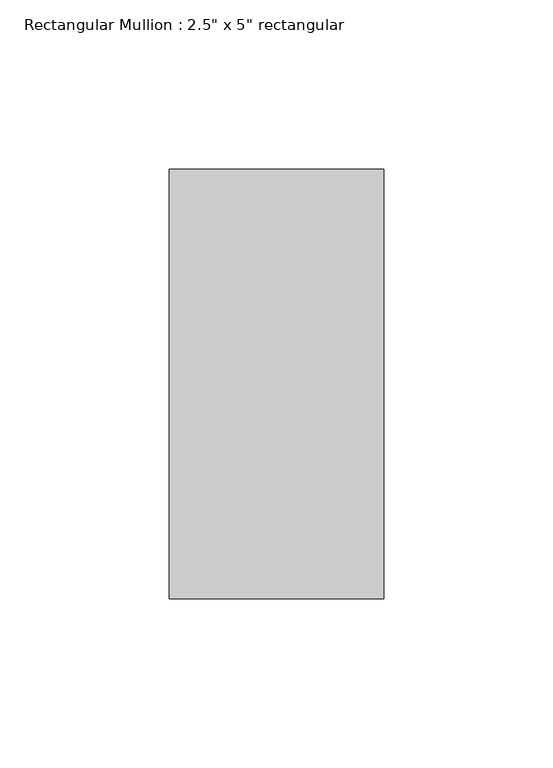
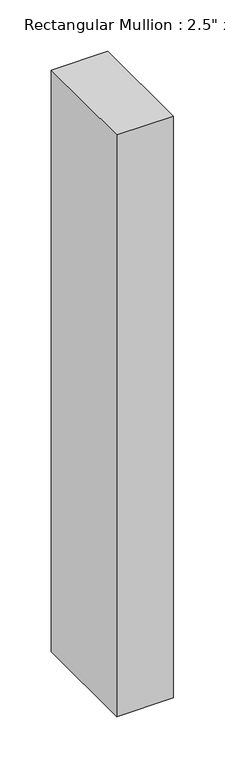
"""IFC4 building model written with IfcOpenShell, lengths in millimetres: member geometry."""

from ifc_helpers import new_model, si_unit, frame, origin, place, context, project, spatial, polyline, outline, extrude, source, transform, mapped, element, save


def member_38fa7f05(model_context):
    return source(origin(), model_context, "Body", "SweptSolid", [
        extrude(outline(polyline([(0.0, 63.5), (0.0, -63.5), (-63.5, -63.5), (-63.5, 63.5), (0.0, 63.5)])), frame((0.0, 0.0, -690.6281505), z_axis=(0.0, 0.0, 1.0), x_axis=(1.0, 0.0, 0.0)), (0.0, 0.0, 1.0), 690.6281505),
    ])


if __name__ == "__main__":
    model = new_model("IFC4")
    model_context = context("Model", 3, world=origin())
    ifc_project = project(units=[si_unit("LENGTHUNIT", "METRE", prefix="MILLI")], contexts=[model_context])
    site = spatial("IfcSite", under=ifc_project)
    building = spatial("IfcBuilding", under=site)
    placement = place(None, origin())
    member_shape = member_38fa7f05(model_context)
    element("IfcMember", 1, ObjectType="Rectangular Mullion : 2.5\" x 5\" rectangular", at=placement, inside=building, context=model_context, shape_type="MappedRepresentation", body=[
        mapped(member_shape, transform((0.0, 0.0, 0.0), x_axis=(1.0, 0.0, 0.0), y_axis=(0.0, 1.0, 0.0), z_axis=(0.0, 0.0, 1.0))),
    ])
    save(model, "model.ifc")

# Revit data of these elements
# Type "Rectangular Mullion : 2.5\" x 5\" rectangular"
#   built-in parameter 1007304 = 0.416667 (stored number, unit not read)
#   built-in parameter 1007301 = 0.104167 (stored number, unit not read)
#   built-in parameter 1007300 = 0.104167 (stored number, unit not read)
# Element 1 (IfcMember, "Rectangular Mullion : 2.5\" x 5\" rectangular")
#   Materials on its faces: "Aluminum"
# Materials
#   "Aluminum": class "Metal", colour RGB 247 247 247, transparency 0, Description = "Aluminum 6061", Cost = 0
